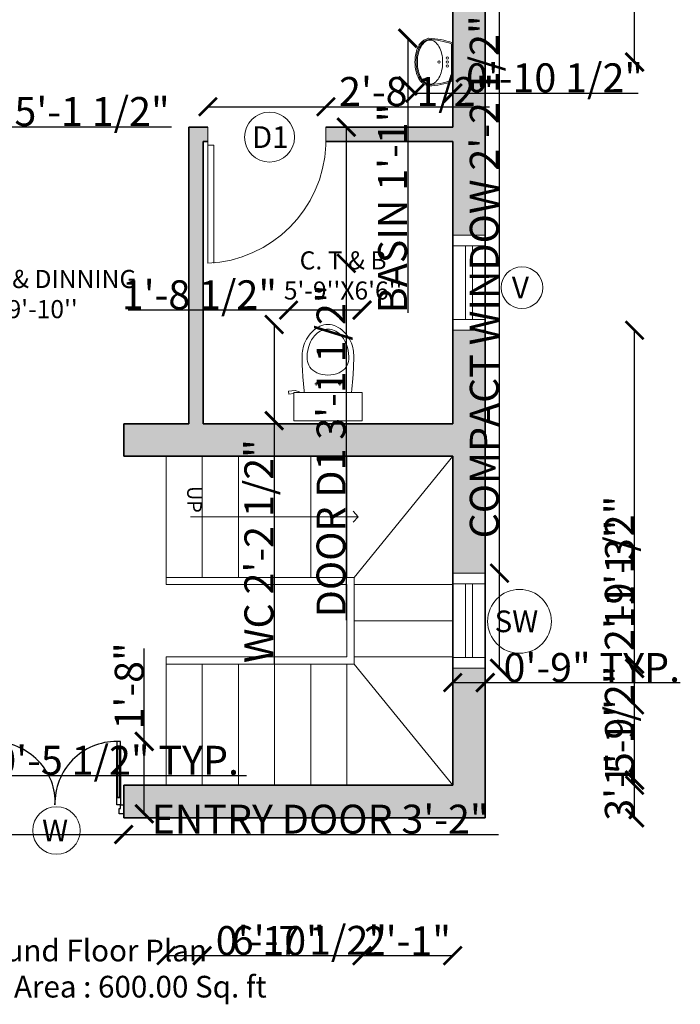
# Model space of a CAD drawing. Units: inches. Extents: x 2163 to 2555, y 1763 to 2232.
# Tile 2 of 3: x 2339 to 2522, y 1763 to 2035. Entities that reach past the tile are written whole.
import ezdxf

# ---------------------------------------------------------------- set-up
doc = ezdxf.new("R2010")
doc.units = ezdxf.units.IN
for name, color, linetype, lineweight in [('A-ANNO-DIMS', 2, 'Continuous', 18), ('A-ANNO-SYMB', 7, 'Continuous', 18), ('A-ANNO-TEXT', 7, 'Continuous', 18), ('A-AREA-IDEN', 7, 'Continuous', 18), ('A-FLOR-FIXT', 9, 'Continuous', 18), ('A-WALL-PATT', 8, 'Continuous', 13), ('Doors', 222, 'Continuous', 18), ('Steps', 50, 'Continuous', 18), ('Walls', 7, 'Continuous', 35), ('Windows', 150, 'Continuous', 18)]:
    doc.layers.add(name, color=color, linetype=linetype, lineweight=lineweight)
doc.layers.add('A-Glaz', color=92, linetype='Continuous')
doc.layers.add('Main Door', color=150, linetype='Continuous')
doc.styles.get("Standard").update_dxf_attribs({"font": 'arial.ttf'})
doc.dimstyles.get("Standard").update_dxf_attribs({"dimtxt": 8, "dimasz": 5, "dimexe": 0.18, "dimexo": 0.0625, "dimgap": 0.09, "dimtad": 1, "dimdec": 1, "dimzin": 0, "dimdsep": 46, "dimlunit": 4, "dimtxsty": 'Standard', "dimblk": 'ARCHTICK', "dimcen": 0.09, "dimse1": 1, "dimse2": 1, "dimadec": 0, "dimazin": 0, "dimtfac": 1, "dimtdec": 1, "dimtofl": 0, "dimtmove": 0, "dimatfit": 3, "dimfxl": 1, "dimtolj": 1, "dimtzin": 0, "dimarcsym": 0})

# ---------------------------------------------------------------- blocks, each defined once
blk = doc.blocks.new('toilet-1')
at = {"color": 0, "linetype": 'ByBlock'}
for p, q in [((-0.23, -0.02), (-0.23, -0.2116)), ((0.23, -0.02), (-0.23, -0.02)), ((0.23, -0.02), (0.23, -0.2116)), ((-0.23, -0.2116), (0.23, -0.2116)), ((-0.0793, -0.2587), (-0.0793, -0.2778)), ((0.0794, -0.2587), (0.0794, -0.2778)), ((0.1917, -0.2144), (0.2206, -0.225)), ((0.2206, -0.225), (0.266, -0.2187)), ((0.2633, -0.1997), (0.23, -0.2044)), ((0.266, -0.2187), (0.2633, -0.1997)), ((-0.0889, -0.2683), (-0.0697, -0.2683)), ((0.0889, -0.2683), (0.0698, -0.2683)), ((0, -0.6382), (0, -0.6382))]:
    blk.add_line(p, q, dxfattribs=at)
for centre, radius, start, end in [((3.5272, -0.6239), 3.7093, 173.69251, 175.15926), ((-3.527, -0.624), 3.7093, 4.84131, 6.31706), ((1.7368, -0.4519), 1.9109, 175.76982, 180.37578), ((0, -0.5169), 0.1884, 66.09393, 113.90607), ((-1.7366, -0.4519), 1.9109, 359.62422, 4.23018), ((-0.0408, -0.4398), 0.0996, 145.14967, 175.88096), ((-0.0312, -0.4465), 0.1114, 113.89968, 145.1485), ((0.0312, -0.4465), 0.1114, 34.8515, 66.10032), ((0.0409, -0.4398), 0.0996, 4.11904, 34.85033), ((0.0353, -0.463), 0.2093, 180.37466, 194.33753), ((0.0981, -0.4497), 0.2389, 175.88621, 195.59308), ((-0.098, -0.4497), 0.2389, 344.40692, 4.11379), ((-0.0351, -0.463), 0.2093, 345.6614, 359.62427), ((0.055, -0.458), 0.2297, 194.33532, 209.62204), ((0.0961, -0.4503), 0.2369, 195.59686, 209.37705), ((-0.096, -0.4503), 0.2369, 330.62295, 344.40314), ((-0.0548, -0.458), 0.2297, 330.37879, 345.66551), ((0.0647, -0.4524), 0.2409, 209.62726, 224.54888), ((0.0232, -0.4913), 0.1532, 209.38715, 226.54376), ((-0.0231, -0.4913), 0.1532, 313.45624, 330.61285), ((-0.0645, -0.4524), 0.2409, 315.45042, 330.37204), ((0.0178, -0.4986), 0.1751, 224.55199, 245.714), ((0.0152, -0.4997), 0.1416, 226.55015, 246.55272), ((0.0004, -0.538), 0.132, 245.58449, 269.87817), ((0, -0.5347), 0.1034, 246.54933, 270.0042), ((0, -0.5347), 0.1034, 269.9958, 293.45067), ((-0.0002, -0.538), 0.132, 270.12162, 294.4153), ((-0.0151, -0.4997), 0.1416, 293.44728, 313.44985), ((-0.0176, -0.4986), 0.1751, 294.28649, 315.4485)]:
    blk.add_arc(centre, radius, start, end, dxfattribs=at)
blk = doc.blocks.new('A$C13CE0A17')
at = {"layer": 'A-Glaz'}
for p, q in [((0.01, 0.61), (0.01, 0.08)), ((0.03, 0.08), (0.03, 0.61))]:
    blk.add_line(p, q, dxfattribs=at)
blk.add_lwpolyline([(1.4, 0.08), (1.4, 0.61), (1.42, 0.61), (1.42, 0.08)], close=True, dxfattribs=at)
at = {"layer": 'Main Door'}
for p, q in [((0, 0.61), (0, 0.69)), ((0, 0.69), (0.04, 0.69)), ((0.04, 0.69), (0.04, 0.61)), ((0, 0.61), (0, 0.08)), ((0.04, 0.61), (0, 0.61)), ((0.04, 0.61), (0, 0.61)), ((0.03, 0.61), (0.01, 0.61)), ((0.04, 0.08), (0.04, 0.61)), ((-0.035, 0), (-0.035, -0.1)), ((0, 0), (-0.035, 0)), ((0, 0.08), (0, 0)), ((0.04, 0.08), (0, 0.08)), ((0, 0.08), (0.04, 0.08)), ((0, 0), (0.04, 0)), ((0, -0.04), (0, 0)), ((0.01, 0.08), (0.03, 0.08)), ((0.04, 0), (0.04, 0.08)), ((-0.035, -0.1), (0.015, -0.1)), ((0.015, -0.04), (0, -0.04)), ((0.015, -0.05), (0.015, -0.04)), ((0.015, -0.1), (0.015, -0.05))]:
    blk.add_line(p, q, dxfattribs=at)
for points in [[(1.39, 0.69), (1.39, 0.61), (1.43, 0.61), (1.43, 0.69)], [(1.39, 0.08), (1.39, 0.61), (1.43, 0.61), (1.43, 0.08)], [(1.39, 0), (1.39, 0.08), (1.43, 0.08), (1.43, 0)], [(1.43, 0), (1.465, 0), (1.465, -0.1), (1.415, -0.1), (1.415, -0.05), (1.415, -0.04), (1.43, -0.04)]]:
    blk.add_lwpolyline(points, close=True, dxfattribs=at)
blk.add_arc((1.387, 0.017), 0.673, 89.7657, 181.4438, dxfattribs=at)
blk.add_ellipse((0.039, 0.051), major_axis=(0.667, -0.122), ratio=0.940794, start_param=0.11153, end_param=1.73917, dxfattribs=at)
blk = doc.blocks.new('AP0B05')
for p, q in [((35, 100), (35, 880)), ((75, 100), (75, 878.9)), ((35, 100), (35, -20)), ((815, 100), (815, -20))]:
    blk.add_line(p, q)
blk.add_lwpolyline([(35, 100), (75, 100)])
blk.add_arc((-2.4, 62.6), 818.3, 2.62122, 87.37878)
blk = doc.blocks.new('wash-3')
at = {"color": 0, "linetype": 'ByBlock'}
blk.add_line((0.23, -0.015), (-0.23, -0.015), dxfattribs=at)
for centre in [(-0.05, -0.066), (0, -0.066), (0.05, -0.066), (0, -0.172)]:
    blk.add_circle(centre, 0.0148, dxfattribs=at)
for centre, radius, start, end in [((0.69, -0.34), 0.991, 159.941, 177.839), ((0.69, -0.34), 0.976, 160.5399, 177.7326), ((-0.69, -0.34), 0.976, 2.2674, 19.4601), ((-0.69, -0.34), 0.991, 2.161, 20.059), ((-0.183, -0.286), 0.095, 144.1588, 180), ((-0.096, -0.349), 0.203, 119.8322, 144.1588), ((-0.038, -0.45), 0.319, 103.3619, 119.8322), ((0, -0.61), 0.483, 90, 103.3619), ((0, -0.61), 0.483, 76.6381, 90), ((0.038, -0.45), 0.319, 60.1678, 76.6381), ((0.096, -0.349), 0.203, 35.8412, 60.1678), ((0.183, -0.286), 0.095, 0, 35.8412), ((-0.12, -0.265), 0.184, 191.7424, 233.4191), ((-0.12, -0.265), 0.169, 192.3358, 233.361), ((-0.183, -0.286), 0.095, 180, 215.8412), ((-0.096, -0.223), 0.203, 215.8412, 240.1678), ((0.096, -0.223), 0.203, 299.8322, 324.1588), ((0.12, -0.265), 0.169, 306.639, 347.6642), ((0.12, -0.265), 0.184, 306.5809, 348.2576), ((0.183, -0.286), 0.095, 324.1588, 0), ((-0.096, -0.223), 0.232, 234.7719, 240.1678), ((-0.096, -0.223), 0.217, 234.8176, 240.1678), ((-0.038, -0.122), 0.348, 240.1678, 256.6381), ((-0.038, -0.122), 0.333, 240.1678, 256.6381), ((-0.038, -0.122), 0.319, 240.1678, 256.6381), ((0, 0.038), 0.513, 256.6381, 270), ((0, 0.038), 0.498, 256.6381, 270), ((0, 0.038), 0.483, 256.6381, 270), ((0, 0.038), 0.483, 270, 283.3619), ((0, 0.038), 0.498, 270, 283.3619), ((0, 0.038), 0.513, 270, 283.3619), ((0.038, -0.122), 0.319, 283.3619, 299.8322), ((0.038, -0.122), 0.333, 283.3619, 299.8322), ((0.038, -0.122), 0.348, 283.3619, 299.8322), ((0.096, -0.223), 0.217, 299.8322, 305.1824), ((0.096, -0.223), 0.232, 299.8322, 305.2281)]:
    blk.add_arc(centre, radius, start, end, dxfattribs=at)
blk = doc.blocks.new('WIN-COMPACT-DOUBLE-FRAME')
for p, q in [((0, 23.32), (9, 23.32)), ((3.5, 3), (3.5, 23.32)), ((5.5, 3), (5.5, 23.32)), ((0, 3), (9, 3))]:
    blk.add_line(p, q)
blk.add_lwpolyline([(0, 0), (0, 26.32), (9, 26.32), (9, 0)], close=True)
blk = doc.blocks.new('TAG-WINDOW-W')
blk.add_circle((6.57, 6.57), 6.57)
blk.add_text('W', height=6).set_placement((2.61, 3.57))
blk = doc.blocks.new('_ArchTick')
at = {"color": 0, "linetype": 'ByBlock', "const_width": 0.15}
blk.add_lwpolyline([(-0.5, -0.5), (0.5, 0.5)], dxfattribs=at)
blk = doc.blocks.new('*D22')
at = {"layer": 'A-ANNO-DIMS', "color": 0, "lineweight": -2, "transparency": 16777216}
for p, q in [((2429.58, 2005.5), (2429.58, 1967.85)), ((2429.58, 1967.85), (2429.58, 1869.14))]:
    blk.add_line(p, q, dxfattribs=at)
at = {"layer": 'Defpoints', "color": 0, "transparency": 16777216}
for p in [(2423.94, 2005.5), (2423.94, 1967.85), (2429.58, 1967.85)]:
    blk.add_point(p, dxfattribs=at)
at = {"layer": 'A-ANNO-DIMS', "color": 0, "lineweight": -2, "transparency": 16777216, "xscale": 5, "yscale": 5, "zscale": 5}
for p, rotation in [((2429.58, 2005.5), 90), ((2429.58, 1967.85), 270)]:
    blk.add_blockref('_ArchTick', p, dxfattribs=dict(at, rotation=rotation))
at = {"layer": 'A-ANNO-DIMS', "color": 0, "transparency": 16777216, "insert": (2425.35, 1915.99), "char_height": 8, "attachment_point": 5, "rotation": 90}
blk.add_mtext('\\A1;DOOR D1 3\'-1 1/2"', dxfattribs=at)
blk = doc.blocks.new('*D23')
at = {"layer": 'A-ANNO-DIMS', "color": 0, "lineweight": -2, "transparency": 16777216}
for p, q in [((2391.3, 2011.15), (2423.94, 2011.15)), ((2423.94, 2011.15), (2469.16, 2011.15))]:
    blk.add_line(p, q, dxfattribs=at)
at = {"layer": 'Defpoints', "color": 0, "transparency": 16777216}
for p in [(2423.94, 2011.15), (2391.3, 2005.5), (2423.94, 2005.5)]:
    blk.add_point(p, dxfattribs=at)
at = {"layer": 'A-ANNO-DIMS', "color": 0, "lineweight": -2, "transparency": 16777216, "xscale": 5, "yscale": 5, "zscale": 5, "rotation": 180}
blk.add_blockref('_ArchTick', (2391.3, 2011.15), dxfattribs=at)
at = {"layer": 'A-ANNO-DIMS', "color": 0, "lineweight": -2, "transparency": 16777216, "xscale": 5, "yscale": 5, "zscale": 5}
blk.add_blockref('_ArchTick', (2423.94, 2011.15), dxfattribs=at)
at = {"layer": 'A-ANNO-DIMS', "color": 0, "transparency": 16777216, "insert": (2449.05, 2015.38), "char_height": 8, "attachment_point": 5}
blk.add_mtext('\\A1;2\'-8 1/2"', dxfattribs=at)
blk = doc.blocks.new('*D24')
at = {"layer": 'A-ANNO-DIMS', "color": 0, "lineweight": -2, "transparency": 16777216}
for p, q in [((2273.83, 1826.19), (2279.47, 1826.19)), ((2279.47, 1826.19), (2402, 1826.19))]:
    blk.add_line(p, q, dxfattribs=at)
at = {"layer": 'Defpoints', "color": 0, "transparency": 16777216}
for p in [(2273.83, 1827.04), (2279.47, 1827.04), (2279.47, 1826.19)]:
    blk.add_point(p, dxfattribs=at)
at = {"layer": 'A-ANNO-DIMS', "color": 0, "lineweight": -2, "transparency": 16777216, "xscale": 5, "yscale": 5, "zscale": 5, "rotation": 180}
blk.add_blockref('_ArchTick', (2273.83, 1826.19), dxfattribs=at)
at = {"layer": 'A-ANNO-DIMS', "color": 0, "lineweight": -2, "transparency": 16777216, "xscale": 5, "yscale": 5, "zscale": 5}
blk.add_blockref('_ArchTick', (2279.47, 1826.19), dxfattribs=at)
at = {"layer": 'A-ANNO-DIMS', "color": 0, "transparency": 16777216, "insert": (2343.23, 1830.42), "char_height": 8, "attachment_point": 5}
blk.add_mtext('\\A1;BURNER 0\'-5 1/2" TYP.', dxfattribs=at)
blk = doc.blocks.new('*D28')
at = {"layer": 'A-ANNO-DIMS', "color": 0, "lineweight": -2, "transparency": 16777216}
for p, q in [((2471.96, 1882.16), (2471.96, 2065.78)), ((2471.96, 1855.84), (2471.96, 1882.16))]:
    blk.add_line(p, q, dxfattribs=at)
at = {"layer": 'Defpoints', "color": 0, "transparency": 16777216}
for p in [(2468.01, 1882.16), (2471.96, 1882.16), (2468.01, 1855.84)]:
    blk.add_point(p, dxfattribs=at)
at = {"layer": 'A-ANNO-DIMS', "color": 0, "lineweight": -2, "transparency": 16777216, "xscale": 5, "yscale": 5, "zscale": 5}
for p, rotation in [((2471.96, 1882.16), 90), ((2471.96, 1855.84), 270)]:
    blk.add_blockref('_ArchTick', p, dxfattribs=dict(at, rotation=rotation))
at = {"layer": 'A-ANNO-DIMS', "color": 0, "transparency": 16777216, "insert": (2467.73, 1976.47), "char_height": 8, "attachment_point": 5, "rotation": 90}
blk.add_mtext('\\A1;COMPACT WINDOW 2\'-2 1/2" TYP.', dxfattribs=at)
blk = doc.blocks.new('*D29')
at = {"layer": 'A-ANNO-DIMS', "color": 0, "lineweight": -2, "transparency": 16777216}
for p, q in [((2459.01, 1851.9), (2468.01, 1851.9)), ((2468.01, 1851.9), (2521.95, 1851.9))]:
    blk.add_line(p, q, dxfattribs=at)
at = {"layer": 'Defpoints', "color": 0, "transparency": 16777216}
for p in [(2459.01, 1855.84), (2468.01, 1855.84), (2468.01, 1851.9)]:
    blk.add_point(p, dxfattribs=at)
at = {"layer": 'A-ANNO-DIMS', "color": 0, "lineweight": -2, "transparency": 16777216, "xscale": 5, "yscale": 5, "zscale": 5, "rotation": 180}
blk.add_blockref('_ArchTick', (2459.01, 1851.9), dxfattribs=at)
at = {"layer": 'A-ANNO-DIMS', "color": 0, "lineweight": -2, "transparency": 16777216, "xscale": 5, "yscale": 5, "zscale": 5}
blk.add_blockref('_ArchTick', (2468.01, 1851.9), dxfattribs=at)
at = {"layer": 'A-ANNO-DIMS', "color": 0, "transparency": 16777216, "insert": (2497.48, 1856.07), "char_height": 8, "attachment_point": 5}
blk.add_mtext('\\A1;0\'-9" TYP.', dxfattribs=at)
blk = doc.blocks.new('*D30')
at = {"layer": 'A-ANNO-DIMS', "color": 0, "lineweight": -2, "transparency": 16777216}
for p, q in [((2409.63, 1950.93), (2409.63, 1924.32)), ((2409.63, 1924.32), (2409.63, 1857.18))]:
    blk.add_line(p, q, dxfattribs=at)
at = {"layer": 'Defpoints', "color": 0, "transparency": 16777216}
for p in [(2413.62, 1950.93), (2409.63, 1924.32), (2413.62, 1924.32)]:
    blk.add_point(p, dxfattribs=at)
at = {"layer": 'A-ANNO-DIMS', "color": 0, "lineweight": -2, "transparency": 16777216, "xscale": 5, "yscale": 5, "zscale": 5}
for p, rotation in [((2409.63, 1950.93), 90), ((2409.63, 1924.32), 270)]:
    blk.add_blockref('_ArchTick', p, dxfattribs=dict(at, rotation=rotation))
at = {"layer": 'A-ANNO-DIMS', "color": 0, "transparency": 16777216, "insert": (2405.4, 1888.25), "char_height": 8, "attachment_point": 5, "rotation": 90}
blk.add_mtext('\\A1;WC 2\'-2 1/2"', dxfattribs=at)
blk = doc.blocks.new('*D31')
at = {"layer": 'A-ANNO-DIMS', "color": 0, "lineweight": -2, "transparency": 16777216}
for p, q in [((2413.62, 1954.92), (2369.29, 1954.92)), ((2433.93, 1954.92), (2413.62, 1954.92))]:
    blk.add_line(p, q, dxfattribs=at)
at = {"layer": 'Defpoints', "color": 0, "transparency": 16777216}
for p in [(2413.62, 1954.92), (2413.62, 1950.93), (2433.93, 1950.93)]:
    blk.add_point(p, dxfattribs=at)
at = {"layer": 'A-ANNO-DIMS', "color": 0, "lineweight": -2, "transparency": 16777216, "xscale": 5, "yscale": 5, "zscale": 5, "rotation": 180}
blk.add_blockref('_ArchTick', (2413.62, 1954.92), dxfattribs=at)
at = {"layer": 'A-ANNO-DIMS', "color": 0, "lineweight": -2, "transparency": 16777216, "xscale": 5, "yscale": 5, "zscale": 5}
blk.add_blockref('_ArchTick', (2433.93, 1954.92), dxfattribs=at)
at = {"layer": 'A-ANNO-DIMS', "color": 0, "transparency": 16777216, "insert": (2388.95, 1959.15), "char_height": 8, "attachment_point": 5}
blk.add_mtext('\\A1;1\'-8 1/2"', dxfattribs=at)
blk = doc.blocks.new('*D32')
at = {"layer": 'A-ANNO-DIMS', "color": 0, "lineweight": -2, "transparency": 16777216}
for p, q in [((2330.01, 1809.91), (2368.01, 1809.91)), ((2368.01, 1809.91), (2471.65, 1809.91))]:
    blk.add_line(p, q, dxfattribs=at)
at = {"layer": 'Defpoints', "color": 0, "transparency": 16777216}
for p in [(2330.01, 1815.61), (2368.01, 1815.61), (2368.01, 1809.91)]:
    blk.add_point(p, dxfattribs=at)
at = {"layer": 'A-ANNO-DIMS', "color": 0, "lineweight": -2, "transparency": 16777216, "xscale": 5, "yscale": 5, "zscale": 5, "rotation": 180}
blk.add_blockref('_ArchTick', (2330.01, 1809.91), dxfattribs=at)
at = {"layer": 'A-ANNO-DIMS', "color": 0, "lineweight": -2, "transparency": 16777216, "xscale": 5, "yscale": 5, "zscale": 5}
blk.add_blockref('_ArchTick', (2368.01, 1809.91), dxfattribs=at)
at = {"layer": 'A-ANNO-DIMS', "color": 0, "transparency": 16777216, "insert": (2422.33, 1814.14), "char_height": 8, "attachment_point": 5}
blk.add_mtext('\\A1;ENTRY DOOR 3\'-2"', dxfattribs=at)
blk = doc.blocks.new('*D33')
at = {"layer": 'A-ANNO-DIMS', "color": 0, "lineweight": -2, "transparency": 16777216}
for p, q in [((2373.71, 1835.64), (2373.71, 1861.34)), ((2373.71, 1815.61), (2373.71, 1835.64))]:
    blk.add_line(p, q, dxfattribs=at)
at = {"layer": 'Defpoints', "color": 0, "transparency": 16777216}
for p in [(2368.01, 1835.64), (2373.71, 1835.64), (2368.01, 1815.61)]:
    blk.add_point(p, dxfattribs=at)
at = {"layer": 'A-ANNO-DIMS', "color": 0, "lineweight": -2, "transparency": 16777216, "xscale": 5, "yscale": 5, "zscale": 5}
for p, rotation in [((2373.71, 1835.64), 90), ((2373.71, 1815.61), 270)]:
    blk.add_blockref('_ArchTick', p, dxfattribs=dict(at, rotation=rotation))
at = {"layer": 'A-ANNO-DIMS', "color": 0, "transparency": 16777216, "insert": (2369.54, 1850.99), "char_height": 8, "attachment_point": 5, "rotation": 90}
blk.add_mtext('\\A1;1\'-8"', dxfattribs=at)
blk = doc.blocks.new('*D38')
at = {"layer": 'A-ANNO-DIMS', "color": 0, "lineweight": -2, "transparency": 16777216}
for p, q in [((2241.35, 2005.61), (2302.62, 2005.61)), ((2302.62, 2005.61), (2381.2, 2005.61))]:
    blk.add_line(p, q, dxfattribs=at)
at = {"layer": 'Defpoints', "color": 0, "transparency": 16777216}
for p in [(2241.35, 2014.8), (2302.62, 2014.8), (2302.62, 2005.61)]:
    blk.add_point(p, dxfattribs=at)
at = {"layer": 'A-ANNO-DIMS', "color": 0, "lineweight": -2, "transparency": 16777216, "xscale": 5, "yscale": 5, "zscale": 5, "rotation": 180}
blk.add_blockref('_ArchTick', (2241.35, 2005.61), dxfattribs=at)
at = {"layer": 'A-ANNO-DIMS', "color": 0, "lineweight": -2, "transparency": 16777216, "xscale": 5, "yscale": 5, "zscale": 5}
blk.add_blockref('_ArchTick', (2302.62, 2005.61), dxfattribs=at)
at = {"layer": 'A-ANNO-DIMS', "color": 0, "transparency": 16777216, "insert": (2344.41, 2009.84), "char_height": 8, "attachment_point": 5}
blk.add_mtext('\\A1;SOFA 5\'-1 1/2"', dxfattribs=at)
blk = doc.blocks.new('*D40')
at = {"layer": 'A-ANNO-DIMS', "color": 0, "lineweight": -2, "transparency": 16777216}
for p, q in [((2446.59, 2030.1), (2446.59, 2016.91)), ((2446.59, 2016.91), (2446.59, 1954.17))]:
    blk.add_line(p, q, dxfattribs=at)
at = {"layer": 'Defpoints', "color": 0, "transparency": 16777216}
for p in [(2448.57, 2030.1), (2446.59, 2016.91), (2448.57, 2016.91)]:
    blk.add_point(p, dxfattribs=at)
at = {"layer": 'A-ANNO-DIMS', "color": 0, "lineweight": -2, "transparency": 16777216, "xscale": 5, "yscale": 5, "zscale": 5}
for p, rotation in [((2446.59, 2030.1), 90), ((2446.59, 2016.91), 270)]:
    blk.add_blockref('_ArchTick', p, dxfattribs=dict(at, rotation=rotation))
at = {"layer": 'A-ANNO-DIMS', "color": 0, "transparency": 16777216, "insert": (2442.37, 1983.04), "char_height": 8, "attachment_point": 5, "rotation": 90}
blk.add_mtext('\\A1;BASIN 1\'-1"', dxfattribs=at)
blk = doc.blocks.new('*D41')
at = {"layer": 'A-ANNO-DIMS', "color": 0, "lineweight": -2, "transparency": 16777216}
for p, q in [((2448.57, 2014.93), (2459.01, 2014.93)), ((2459.01, 2014.93), (2510.31, 2014.93))]:
    blk.add_line(p, q, dxfattribs=at)
at = {"layer": 'Defpoints', "color": 0, "transparency": 16777216}
for p in [(2448.57, 2016.91), (2459.01, 2016.91), (2459.01, 2014.93)]:
    blk.add_point(p, dxfattribs=at)
at = {"layer": 'A-ANNO-DIMS', "color": 0, "lineweight": -2, "transparency": 16777216, "xscale": 5, "yscale": 5, "zscale": 5, "rotation": 180}
blk.add_blockref('_ArchTick', (2448.57, 2014.93), dxfattribs=at)
at = {"layer": 'A-ANNO-DIMS', "color": 0, "lineweight": -2, "transparency": 16777216, "xscale": 5, "yscale": 5, "zscale": 5}
blk.add_blockref('_ArchTick', (2459.01, 2014.93), dxfattribs=at)
at = {"layer": 'A-ANNO-DIMS', "color": 0, "transparency": 16777216, "insert": (2487.16, 2019.16), "char_height": 8, "attachment_point": 5}
blk.add_mtext('\\A1;0\'-10 1/2"', dxfattribs=at)
blk = doc.blocks.new('*D49')
at = {"layer": 'A-ANNO-DIMS', "color": 0, "lineweight": -2, "transparency": 16777216}
blk.add_line((2509.31, 1814.5), (2509.31, 1855.84), dxfattribs=at)
at = {"layer": 'Defpoints', "color": 0, "transparency": 16777216}
for p in [(2468.01, 1855.84), (2509.31, 1855.84), (2468.01, 1814.5)]:
    blk.add_point(p, dxfattribs=at)
at = {"layer": 'A-ANNO-DIMS', "color": 0, "lineweight": -2, "transparency": 16777216, "xscale": 5, "yscale": 5, "zscale": 5}
for p, rotation in [((2509.31, 1855.84), 90), ((2509.31, 1814.5), 270)]:
    blk.add_blockref('_ArchTick', p, dxfattribs=dict(at, rotation=rotation))
at = {"layer": 'A-ANNO-DIMS', "color": 0, "transparency": 16777216, "insert": (2505.09, 1835.17), "char_height": 8, "attachment_point": 5, "rotation": 90}
blk.add_mtext('\\A1;3\'-5 1/2"', dxfattribs=at)
blk = doc.blocks.new('*D50')
at = {"layer": 'A-ANNO-DIMS', "color": 0, "lineweight": -2, "transparency": 16777216}
blk.add_line((2509.31, 1814.5), (2509.31, 1949.34), dxfattribs=at)
at = {"layer": 'Defpoints', "color": 0, "transparency": 16777216}
for p in [(2468.01, 1949.34), (2509.31, 1949.34), (2468.01, 1814.5)]:
    blk.add_point(p, dxfattribs=at)
at = {"layer": 'A-ANNO-DIMS', "color": 0, "lineweight": -2, "transparency": 16777216, "xscale": 5, "yscale": 5, "zscale": 5}
for p, rotation in [((2509.31, 1949.34), 90), ((2509.31, 1814.5), 270)]:
    blk.add_blockref('_ArchTick', p, dxfattribs=dict(at, rotation=rotation))
at = {"layer": 'A-ANNO-DIMS', "color": 0, "transparency": 16777216, "insert": (2505.14, 1881.92), "char_height": 8, "attachment_point": 5, "rotation": 90}
blk.add_mtext('\\A1;11\'-3"', dxfattribs=at)
blk = doc.blocks.new('*D52')
at = {"layer": 'A-ANNO-DIMS', "color": 0, "lineweight": -2, "transparency": 16777216}
blk.add_line((2379.73, 1776.39), (2459.01, 1776.39), dxfattribs=at)
at = {"layer": 'Defpoints', "color": 0, "transparency": 16777216}
for p in [(2379.73, 1823.5), (2459.01, 1823.5), (2459.01, 1776.39)]:
    blk.add_point(p, dxfattribs=at)
at = {"layer": 'A-ANNO-DIMS', "color": 0, "lineweight": -2, "transparency": 16777216, "xscale": 5, "yscale": 5, "zscale": 5, "rotation": 180}
blk.add_blockref('_ArchTick', (2379.73, 1776.39), dxfattribs=at)
at = {"layer": 'A-ANNO-DIMS', "color": 0, "lineweight": -2, "transparency": 16777216, "xscale": 5, "yscale": 5, "zscale": 5}
blk.add_blockref('_ArchTick', (2459.01, 1776.39), dxfattribs=at)
at = {"layer": 'A-ANNO-DIMS', "color": 0, "transparency": 16777216, "insert": (2419.37, 1780.62), "char_height": 8, "attachment_point": 5}
blk.add_mtext('\\A1;6\'-7 1/2"', dxfattribs=at)
blk = doc.blocks.new('*D53')
at = {"layer": 'A-ANNO-DIMS', "color": 0, "lineweight": -2, "transparency": 16777216}
for p, q in [((2509.31, 1857), (2509.31, 1902.23)), ((2509.31, 1823.5), (2509.31, 1857))]:
    blk.add_line(p, q, dxfattribs=at)
at = {"layer": 'Defpoints', "color": 0, "transparency": 16777216}
for p in [(2431.73, 1857), (2509.31, 1857), (2459.01, 1823.5)]:
    blk.add_point(p, dxfattribs=at)
at = {"layer": 'A-ANNO-DIMS', "color": 0, "lineweight": -2, "transparency": 16777216, "xscale": 5, "yscale": 5, "zscale": 5}
for p, rotation in [((2509.31, 1857), 90), ((2509.31, 1823.5), 270)]:
    blk.add_blockref('_ArchTick', p, dxfattribs=dict(at, rotation=rotation))
at = {"layer": 'A-ANNO-DIMS', "color": 0, "transparency": 16777216, "insert": (2505.09, 1882.12), "char_height": 8, "attachment_point": 5, "rotation": 90}
blk.add_mtext('\\A1;2\'-9 1/2"', dxfattribs=at)
blk = doc.blocks.new('*D54')
at = {"layer": 'A-ANNO-DIMS', "color": 0, "lineweight": -2, "transparency": 16777216}
for p, q in [((2379.73, 1776.39), (2389.73, 1776.39)), ((2389.73, 1776.39), (2422.39, 1776.39))]:
    blk.add_line(p, q, dxfattribs=at)
at = {"layer": 'Defpoints', "color": 0, "transparency": 16777216}
for p in [(2379.73, 1823.5), (2389.73, 1823.5), (2389.73, 1776.39)]:
    blk.add_point(p, dxfattribs=at)
at = {"layer": 'A-ANNO-DIMS', "color": 0, "lineweight": -2, "transparency": 16777216, "xscale": 5, "yscale": 5, "zscale": 5, "rotation": 180}
blk.add_blockref('_ArchTick', (2379.73, 1776.39), dxfattribs=at)
at = {"layer": 'A-ANNO-DIMS', "color": 0, "lineweight": -2, "transparency": 16777216, "xscale": 5, "yscale": 5, "zscale": 5}
blk.add_blockref('_ArchTick', (2389.73, 1776.39), dxfattribs=at)
at = {"layer": 'A-ANNO-DIMS', "color": 0, "transparency": 16777216, "insert": (2408.56, 1780.56), "char_height": 8, "attachment_point": 5}
blk.add_mtext('\\A1;0\'-10"', dxfattribs=at)
blk = doc.blocks.new('*D56')
at = {"layer": 'A-ANNO-DIMS', "color": 0, "lineweight": -2, "transparency": 16777216}
blk.add_line((2433.93, 1776.39), (2459.01, 1776.39), dxfattribs=at)
at = {"layer": 'Defpoints', "color": 0, "transparency": 16777216}
for p in [(2433.93, 1924.32), (2459.01, 1923.5), (2459.01, 1776.39)]:
    blk.add_point(p, dxfattribs=at)
at = {"layer": 'A-ANNO-DIMS', "color": 0, "lineweight": -2, "transparency": 16777216, "xscale": 5, "yscale": 5, "zscale": 5, "rotation": 180}
blk.add_blockref('_ArchTick', (2433.93, 1776.39), dxfattribs=at)
at = {"layer": 'A-ANNO-DIMS', "color": 0, "lineweight": -2, "transparency": 16777216, "xscale": 5, "yscale": 5, "zscale": 5}
blk.add_blockref('_ArchTick', (2459.01, 1776.39), dxfattribs=at)
at = {"layer": 'A-ANNO-DIMS', "color": 0, "transparency": 16777216, "insert": (2446.47, 1780.5), "char_height": 8, "attachment_point": 5}
blk.add_mtext('\\A1;2\'-1"', dxfattribs=at)
blk = doc.blocks.new('*D57')
at = {"layer": 'A-ANNO-DIMS', "color": 0, "lineweight": -2, "transparency": 16777216}
for p, q in [((2509.31, 2041.5), (2509.31, 2067.2)), ((2509.31, 2023.5), (2509.31, 2041.5))]:
    blk.add_line(p, q, dxfattribs=at)
at = {"layer": 'Defpoints', "color": 0, "transparency": 16777216}
for p in [(2459.01, 2041.5), (2509.31, 2041.5), (2459.84, 2023.5)]:
    blk.add_point(p, dxfattribs=at)
at = {"layer": 'A-ANNO-DIMS', "color": 0, "lineweight": -2, "transparency": 16777216, "xscale": 5, "yscale": 5, "zscale": 5}
for p, rotation in [((2509.31, 2041.5), 90), ((2509.31, 2023.5), 270)]:
    blk.add_blockref('_ArchTick', p, dxfattribs=dict(at, rotation=rotation))
at = {"layer": 'A-ANNO-DIMS', "color": 0, "transparency": 16777216, "insert": (2505.14, 2056.85), "char_height": 8, "attachment_point": 5, "rotation": 90}
blk.add_mtext('\\A1;1\'-6"', dxfattribs=at)
blk = doc.blocks.new('*D59')
at = {"layer": 'A-ANNO-DIMS', "color": 0, "lineweight": -2, "transparency": 16777216}
blk.add_line((2509.31, 1824.94), (2509.31, 1845.73), dxfattribs=at)
at = {"layer": 'Defpoints', "color": 0, "transparency": 16777216}
for p in [(2278.7, 1845.73), (2509.31, 1845.73), (2278.7, 1824.94)]:
    blk.add_point(p, dxfattribs=at)
at = {"layer": 'A-ANNO-DIMS', "color": 0, "lineweight": -2, "transparency": 16777216, "xscale": 5, "yscale": 5, "zscale": 5}
for p, rotation in [((2509.31, 1845.73), 90), ((2509.31, 1824.94), 270)]:
    blk.add_blockref('_ArchTick', p, dxfattribs=dict(at, rotation=rotation))
at = {"layer": 'A-ANNO-DIMS', "color": 0, "transparency": 16777216, "insert": (2505.14, 1835.33), "char_height": 8, "attachment_point": 5, "rotation": 90}
blk.add_mtext('\\A1;1\'-9"', dxfattribs=at)

msp = doc.modelspace()

# ---------------------------------------------------------------- hatches: boundary and pattern name
at = {"layer": 'A-WALL-PATT', "transparency": 33554585}
h = msp.add_hatch(color=256, dxfattribs=at)
h.dxf.hatch_style = 1
h.paths.add_polyline_path([(2261.51, 2174.5), (2228.01, 2174.5), (2228.01, 2135.5), (2237.01, 2135.5), (2237.01, 2165.5), (2261.51, 2165.5)])
h.paths.add_polyline_path([(2237.01, 2075.5), (2228.01, 2075.5), (2228.01, 2012.5), (2237.01, 2012.5), (2237.01, 2041.5), (2306.96, 2041.5), (2306.96, 2045.5), (2237.01, 2045.5)])
h.paths.add_polyline_path([(2237.01, 1952.5), (2228.01, 1952.5), (2228.01, 1901.5), (2237.01, 1901.5), (2237.01, 1919.5), (2281.23, 1919.5), (2281.23, 1923.5), (2237.01, 1923.5)])
h.paths.add_polyline_path([(2237.01, 1841.5), (2228.01, 1841.5), (2228.01, 1814.5), (2249.01, 1814.5), (2249.01, 1823.5), (2237.01, 1823.5)])
h.paths.add_polyline_path([(2330.01, 1923.5), (2320.02, 1923.5), (2320.02, 1919.5), (2321.01, 1919.5), (2321.01, 1823.5), (2309.01, 1823.5), (2309.01, 1814.5), (2330.01, 1814.5)])
h.paths.add_polyline_path([(2468.01, 1855.84), (2459.01, 1855.84), (2459.01, 1823.5), (2368.01, 1823.5), (2368.01, 1814.5), (2468.01, 1814.5)])
h.paths.add_polyline_path([(2468.01, 1949.34), (2459.01, 1949.34), (2459.01, 1923.5), (2390.01, 1923.5), (2390.01, 2001.5), (2391.3, 2001.5), (2391.3, 2005.5), (2386.01, 2005.5), (2386.01, 1923.5), (2368.01, 1923.5), (2368.01, 1914.5), (2459.01, 1914.5), (2459.01, 1882.16), (2468.01, 1882.16)])
h.paths.add_polyline_path([(2468.01, 2077.97), (2459.01, 2077.97), (2459.01, 2045.5), (2389.06, 2045.5), (2389.06, 2041.5), (2459.01, 2041.5), (2459.01, 2005.5), (2423.94, 2005.5), (2423.94, 2001.5), (2459.01, 2001.5), (2459.01, 1975.66), (2468.01, 1975.66)])
h.paths.add_polyline_path([(2468.01, 2174.5), (2434.51, 2174.5), (2434.51, 2165.5), (2450.4, 2165.5), (2459.01, 2165.5), (2459.01, 2137.97), (2468.01, 2137.97)])

# ---------------------------------------------------------------- linework, layer by layer
at = {"layer": 'A-ANNO-SYMB'}
for p, q in [((2432.89, 1897.75), (2431.48, 1899.27)), ((2386.5, 1897.75), (2432.89, 1897.75)), ((2432.89, 1897.75), (2431.48, 1896.23))]:
    msp.add_line(p, q, dxfattribs=at)
for centre, radius in [((2408.37, 2002.77), 6.9), ((2478.16, 1961.13), 5.76), ((2477.48, 1868.84), 8.83)]:
    msp.add_circle(centre, radius, dxfattribs=at)
at = {"layer": 'Steps'}
for p, q in [((2379.73, 1879), (2379.73, 1914.5)), ((2389.73, 1881), (2389.73, 1914.5)), ((2399.73, 1881), (2399.73, 1914.5)), ((2409.73, 1881), (2409.73, 1914.5)), ((2419.73, 1881), (2419.73, 1914.5)), ((2429.73, 1881), (2429.73, 1914.5)), ((2431.73, 1881), (2459.01, 1914.5)), ((2431.73, 1881), (2379.73, 1881)), ((2429.73, 1879), (2379.73, 1879)), ((2429.73, 1859), (2429.73, 1879)), ((2431.73, 1857), (2431.73, 1881)), ((2431.73, 1879), (2459.01, 1879)), ((2431.73, 1869), (2459.01, 1869)), ((2379.73, 1823.5), (2379.73, 1859)), ((2429.73, 1859), (2379.73, 1859)), ((2431.73, 1859), (2459.01, 1859)), ((2431.73, 1857), (2379.73, 1857)), ((2389.73, 1823.5), (2389.73, 1857)), ((2399.73, 1823.5), (2399.73, 1857)), ((2409.73, 1823.5), (2409.73, 1857)), ((2419.73, 1823.5), (2419.73, 1857)), ((2429.73, 1823.5), (2429.73, 1857)), ((2431.73, 1857), (2459.01, 1823.5))]:
    msp.add_line(p, q, dxfattribs=at)
at = {"layer": 'Walls'}
for p, q in [((2468.01, 2174.5), (2468.01, 1814.5)), ((2459.01, 2041.5), (2459.01, 2005.5)), ((2386.01, 2005.5), (2386.01, 1923.5)), ((2386.01, 2005.5), (2391.3, 2005.5)), ((2423.94, 2005.5), (2459.01, 2005.5)), ((2390.01, 2001.5), (2390.01, 1923.5)), ((2390.01, 2001.5), (2391.3, 2001.5)), ((2423.94, 2001.5), (2459.01, 2001.5)), ((2459.01, 2001.5), (2459.01, 1923.5)), ((2368.01, 1923.5), (2386.01, 1923.5)), ((2368.01, 1923.5), (2368.01, 1914.5)), ((2390.01, 1923.5), (2459.01, 1923.5)), ((2368.01, 1914.5), (2459.01, 1914.5)), ((2459.01, 1914.5), (2459.01, 1823.5)), ((2368.01, 1823.5), (2368.01, 1814.5)), ((2368.01, 1823.5), (2459.01, 1823.5)), ((2368.01, 1814.5), (2468.01, 1814.5))]:
    msp.add_line(p, q, dxfattribs=at)

# ---------------------------------------------------------------- block references
at = {"layer": 'A-ANNO-SYMB'}
msp.add_blockref('TAG-WINDOW-W', (2342.84, 1804.43), dxfattribs=at)
at = {"layer": 'A-FLOR-FIXT'}
for name, p, xscale, yscale, zscale, rotation in [('wash-3', (2459.01, 2023.5), 21.97868668078204, 21.97868668078204, 21.97868668078204, 270), ('toilet-1', (2424.51, 1923.5), 40.93443561245635, 40.93443561245635, 40.93443561245635, 180)]:
    msp.add_blockref(name, p, dxfattribs=dict(at, xscale=xscale, yscale=yscale, zscale=zscale, rotation=rotation))
at = {"layer": 'Doors', "xscale": -0.0418353091341889, "yscale": 0.0418353091341889, "zscale": 0.0418353091341889, "rotation": 180}
msp.add_blockref('AP0B05', (2389.84, 2004.67), dxfattribs=at)
at = {"layer": 'Doors', "xscale": 25.33333333333333, "yscale": 25.33333333333333, "zscale": 25.33333333333333}
msp.add_blockref('A$C13CE0A17', (2330.9, 1818.14), dxfattribs=at)
at = {"layer": 'Windows'}
for p in [(2459.01, 1949.35), (2459.01, 1855.85)]:
    msp.add_blockref('WIN-COMPACT-DOUBLE-FRAME', p, dxfattribs=at)

# ---------------------------------------------------------------- texts
at = {"layer": 'A-ANNO-SYMB'}
for s, p in [('D1', (2403.46, 1999.76)), ('V', (2475.38, 1958.13)), ('SW', (2470.59, 1865.84))]:
    msp.add_text(s, height=6, dxfattribs=at).set_placement(p)
at = {"layer": 'A-ANNO-TEXT'}
msp.add_text('UP', height=4, rotation=270, dxfattribs=at).set_placement((2385.58, 1906.25))
at = {"layer": 'A-ANNO-TEXT', "insert": (2275.16, 1780.81), "char_height": 6, "attachment_point": 1}
msp.add_mtext_dynamic_manual_height_columns('\\pxqc;Ground Floor Plan\\PBuilt Up Area : 600.00 Sq. ft', width=162.2537, gutter_width=78.9, heights=[32.47], dxfattribs=at)
at = {"layer": 'A-AREA-IDEN', "char_height": 5, "attachment_point": 1}
for s, width, heights, insert in [("\\pxqc;C. T & B\\P5'-9''X6'6''", 40.594, [0], (2408.4, 1971.17)), ("\\pxqc;LIVING HALL & DINNING\\P12'-5''X9'-10''", 82.4336, [20.1], (2292.72, 1966.02))]:
    msp.add_mtext_dynamic_manual_height_columns(s, width=width, gutter_width=12.5, heights=heights, dxfattribs=dict(at, insert=insert))

# ---------------------------------------------------------------- dimensions: what is measured, and where the dimension line sits
at = {"layer": 'A-ANNO-DIMS'}
for base, p1, p2, angle, picture, middle in [((2509.31, 2041.5), (2459.84, 2023.5), (2459.01, 2041.5), 90, '*D57', (2505.14, 2056.85)), ((2413.62, 1954.92), (2433.93, 1950.93), (2413.62, 1950.93), 180, '*D31', (2388.95, 1959.15)), ((2509.31, 1949.34), (2468.01, 1814.5), (2468.01, 1949.34), 90, '*D50', (2505.14, 1881.92)), ((2509.31, 1857), (2459.01, 1823.5), (2431.73, 1857), 90, '*D53', (2505.09, 1882.12)), ((2373.71, 1835.64), (2368.01, 1815.61), (2368.01, 1835.64), 90, '*D33', (2369.54, 1850.99)), ((2509.31, 1855.84), (2468.01, 1814.5), (2468.01, 1855.84), 90, '*D49', (2505.09, 1835.17)), ((2509.31, 1845.73), (2278.7, 1824.94), (2278.7, 1845.73), 90, '*D59', (2505.14, 1835.33))]:
    dim = msp.add_linear_dim(base=base, p1=p1, p2=p2, angle=angle, dimstyle='Standard', override={"dimdec": 1, "dimlfac": 1, "dimrnd": 0, "dimzin": 1, "dimdsep": 46, "dimlunit": 4, "dimfrac": 2}, dxfattribs=at)
    dim.commit()
    dim.dimension.update_dxf_attribs({"geometry": picture, "text_midpoint": middle})
for base, p1, p2, angle, text, picture, middle in [((2471.96, 1882.16), (2468.01, 1855.84), (2468.01, 1882.16), 90, 'COMPACT WINDOW <> TYP.', '*D28', (2467.73, 1976.47)), ((2446.59, 2016.91), (2448.57, 2030.1), (2448.57, 2016.91), 270, 'BASIN <>', '*D40', (2442.37, 1983.04)), ((2429.5828, 1967.8516), (2423.9351, 2005.5033), (2423.9351, 1967.8516), 270, 'DOOR D1 <>', '*D22', (2425.351, 1915.9948)), ((2409.63, 1924.32), (2413.62, 1950.93), (2413.62, 1924.32), 270, 'WC <>', '*D30', (2405.4, 1888.25))]:
    dim = msp.add_linear_dim(base=base, p1=p1, p2=p2, angle=angle, text=text, dimstyle='Standard', override={"dimdec": 1, "dimlfac": 1, "dimrnd": 0, "dimzin": 1, "dimdsep": 46, "dimlunit": 4, "dimfrac": 2}, dxfattribs=at)
    dim.commit()
    dim.dimension.update_dxf_attribs({"geometry": picture, "text_midpoint": middle})
for base, p1, p2, picture, middle in [((2459.01, 2014.93), (2448.57, 2016.91), (2459.01, 2016.91), '*D41', (2487.16, 2019.16)), ((2423.94, 2011.15), (2391.3, 2005.5), (2423.94, 2005.5), '*D23', (2449.05, 2015.38)), ((2459.01, 1776.39), (2433.93, 1924.32), (2459.01, 1923.5), '*D56', (2446.47, 1780.5)), ((2459.01, 1776.39), (2379.73, 1823.5), (2459.01, 1823.5), '*D52', (2419.37, 1780.62)), ((2389.73, 1776.39), (2379.73, 1823.5), (2389.73, 1823.5), '*D54', (2408.56, 1780.56))]:
    dim = msp.add_linear_dim(base=base, p1=p1, p2=p2, dimstyle='Standard', override={"dimdec": 1, "dimlfac": 1, "dimrnd": 0, "dimzin": 1, "dimdsep": 46, "dimlunit": 4, "dimfrac": 2}, dxfattribs=at)
    dim.commit()
    dim.dimension.update_dxf_attribs({"geometry": picture, "text_midpoint": middle})
for base, p1, p2, text, picture, middle in [((2302.62, 2005.61), (2241.35, 2014.8), (2302.62, 2014.8), 'SOFA <>', '*D38', (2344.41, 2009.84)), ((2468.01, 1851.9), (2459.01, 1855.84), (2468.01, 1855.84), '<> TYP.', '*D29', (2497.48, 1856.07)), ((2279.47, 1826.19), (2273.83, 1827.04), (2279.47, 1827.04), 'BURNER <> TYP.', '*D24', (2343.23, 1830.42)), ((2368.01, 1809.91), (2330.01, 1815.61), (2368.01, 1815.61), 'ENTRY DOOR <>', '*D32', (2422.33, 1814.14))]:
    dim = msp.add_linear_dim(base=base, p1=p1, p2=p2, text=text, dimstyle='Standard', override={"dimdec": 1, "dimlfac": 1, "dimrnd": 0, "dimzin": 1, "dimdsep": 46, "dimlunit": 4, "dimfrac": 2}, dxfattribs=at)
    dim.commit()
    dim.dimension.update_dxf_attribs({"geometry": picture, "text_midpoint": middle})

doc.saveas('drawing.dxf')
